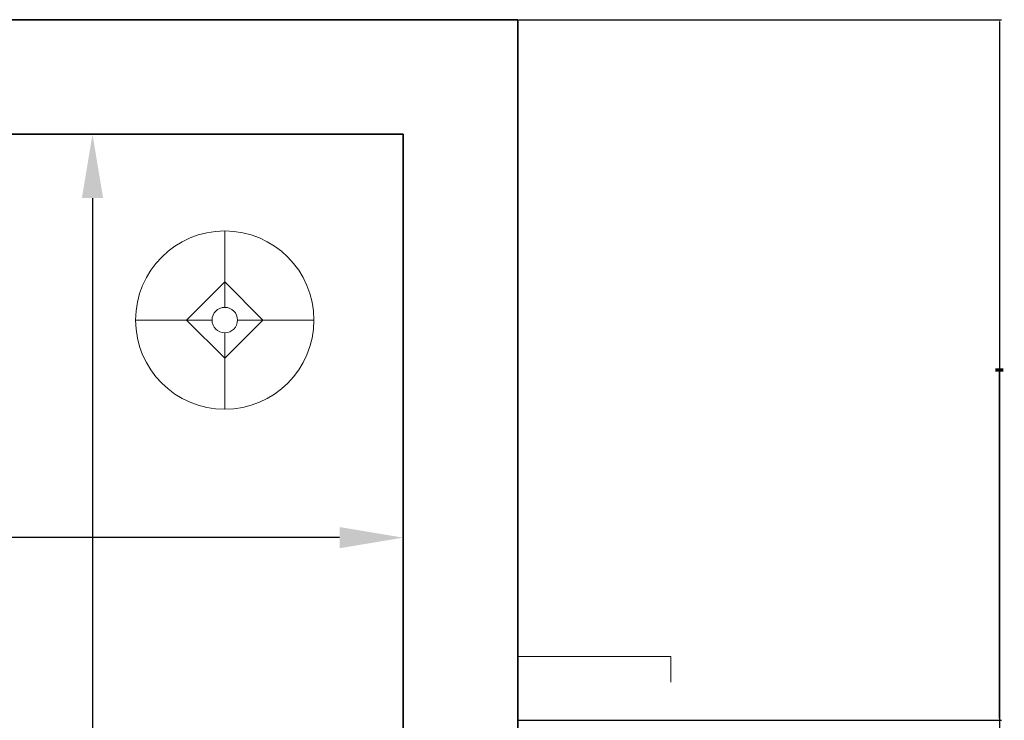
# Model space of a CAD drawing. Units: inches. Extents: x -128 to 854, y -395 to 398.
# Tile 49 of 61: x 275 to 352, y 294 to 349. Entities that reach past the tile are written whole.
import ezdxf

# ---------------------------------------------------------------- set-up
doc = ezdxf.new("R2010")
doc.units = ezdxf.units.IN
doc.header["$MEASUREMENT"] = 0
doc.linetypes.add('ACAD_ISO02W100', pattern=[15, 12, -3])
for name, color, linetype, lineweight in [('A-ANNO-DIMS', 2, 'Continuous', 18), ('A-FURN', 8, 'Continuous', 18), ('A-GLAZ-OVHD', 220, 'ACAD_ISO02W100', 13), ('A-WALL', 4, 'Continuous', 35)]:
    doc.layers.add(name, color=color, linetype=linetype, lineweight=lineweight)
doc.styles.get("Standard").update_dxf_attribs({"font": 'arial.ttf'})
doc.dimstyles.get("Standard").update_dxf_attribs({"dimtxt": 0.18, "dimasz": 0.18, "dimexe": 0.18, "dimexo": 0.0625, "dimgap": 0.09, "dimtad": 0, "dimtih": 1, "dimtoh": 1, "dimdec": 1, "dimzin": 0, "dimdsep": 46, "dimlunit": 4, "dimtxsty": 'Standard', "dimcen": 0.09, "dimclrd": 1, "dimclre": 2, "dimclrt": 6, "dimadec": 0, "dimazin": 0, "dimtfac": 1, "dimtdec": 1, "dimtofl": 0, "dimtmove": 0, "dimatfit": 3, "dimfxl": 1, "dimtfill": 2, "dimtfillclr": 3, "dimtolj": 1, "dimtzin": 0, "dimarcsym": 0})

# ---------------------------------------------------------------- blocks, each defined once
blk = doc.blocks.new('Lamp - Table')
for p, q in [((0, 7), (0, 1)), ((0, 3), (-3, 0)), ((3, 0), (0, 3)), ((-1, 0), (-7, 0)), ((-3, 0), (0, -3)), ((0, -3), (3, 0)), ((1, 0), (7, 0)), ((0, -1), (0, -7))]:
    blk.add_line(p, q)
for radius in [7, 1]:
    blk.add_circle((0, 0), radius)
blk = doc.blocks.new('*D52')
at = {"layer": 'A-ANNO-DIMS', "color": 0, "lineweight": -2, "transparency": 16777216}
for p, q in [((180.873, 339.678), (180.873, 307.9)), ((304.873, 339.678), (304.873, 307.9)), ((185.873, 308.08), (236.101, 308.08)), ((299.873, 308.08), (249.645, 308.08))]:
    blk.add_line(p, q, dxfattribs=at)
at = {"layer": 'A-ANNO-DIMS', "color": 0, "transparency": 16777216}
for points in [[(185.873, 308.913), (185.873, 307.247), (180.873, 308.08)], [(299.873, 308.913), (299.873, 307.247), (304.873, 308.08)]]:
    blk.add_solid(points, dxfattribs=at)
at = {"layer": 'Defpoints', "color": 0, "transparency": 16777216}
for p in [(180.873, 339.741), (304.873, 339.741), (304.873, 308.08)]:
    blk.add_point(p, dxfattribs=at)
at = {"layer": 'A-ANNO-DIMS', "color": 0, "transparency": 16777216, "insert": (242.873, 308.08), "char_height": 4, "attachment_point": 5, "bg_fill": 1, "box_fill_scale": 1.25, "bg_fill_color": 3, "bg_fill_transparency": 0}
blk.add_mtext('\\A1;10\'-4"', dxfattribs=at)
blk = doc.blocks.new('*D53')
at = {"layer": 'A-ANNO-DIMS', "color": 0, "lineweight": -2, "transparency": 16777216}
for p, q in [((304.81, 339.741), (280.297, 339.741)), ((280.477, 334.741), (280.477, 269.839)), ((280.477, 200.741), (280.477, 265.642)), ((304.81, 195.741), (280.297, 195.741))]:
    blk.add_line(p, q, dxfattribs=at)
at = {"layer": 'A-ANNO-DIMS', "color": 0, "transparency": 16777216}
for points in [[(279.644, 334.741), (281.311, 334.741), (280.477, 339.741)], [(279.644, 200.741), (281.311, 200.741), (280.477, 195.741)]]:
    blk.add_solid(points, dxfattribs=at)
at = {"layer": 'Defpoints', "color": 0, "transparency": 16777216}
for p in [(280.477, 339.741), (304.873, 339.741), (304.873, 195.741)]:
    blk.add_point(p, dxfattribs=at)
at = {"layer": 'A-ANNO-DIMS', "color": 0, "transparency": 16777216, "insert": (280.477, 267.741), "char_height": 4, "attachment_point": 5, "bg_fill": 1, "box_fill_scale": 1.25, "bg_fill_color": 3, "bg_fill_transparency": 0}
blk.add_mtext("\\A1;12'", dxfattribs=at)
blk = doc.blocks.new('SHADE-48IN')
at = {"ltscale": 2}
for p, q in [((12, 62), (0, 62)), ((0, 0), (0, 62)), ((12, 57), (12, 62)), ((12, 5), (12, 0)), ((12, 0), (0, 0))]:
    blk.add_line(p, q, dxfattribs=at)
blk = doc.blocks.new('*D98')
at = {"layer": 'A-ANNO-DIMS', "color": 2, "lineweight": -2, "transparency": 16777216}
for p, q in [((313.935, 348.741), (351.853, 348.741)), ((313.935, -89.259), (351.853, -89.259))]:
    blk.add_line(p, q, dxfattribs=at)
at = {"layer": 'A-ANNO-DIMS', "color": 1, "lineweight": -2, "transparency": 16777216}
for p, q in [((351.673, 348.561), (351.673, 129.923)), ((351.673, -89.079), (351.673, 129.559))]:
    blk.add_line(p, q, dxfattribs=at)
at = {"layer": 'A-ANNO-DIMS', "color": 1, "transparency": 16777216}
for points in [[(351.643, 348.561), (351.703, 348.561), (351.673, 348.741)], [(351.643, -89.079), (351.703, -89.079), (351.673, -89.259)]]:
    blk.add_solid(points, dxfattribs=at)
at = {"layer": 'Defpoints', "color": 0, "transparency": 16777216}
for p in [(313.873, 348.741), (351.673, 348.741), (313.873, -89.259)]:
    blk.add_point(p, dxfattribs=at)
at = {"layer": 'A-ANNO-DIMS', "color": 6, "transparency": 16777216, "insert": (351.673, 129.741), "char_height": 0.18, "attachment_point": 5, "bg_fill": 1, "box_fill_scale": 1.25, "bg_fill_color": 3, "bg_fill_transparency": 0}
blk.add_mtext('\\A1;36\'-6"', dxfattribs=at)
blk = doc.blocks.new('*D113')
at = {"layer": 'A-ANNO-DIMS', "color": 2, "lineweight": -2, "transparency": 16777216}
for p, q in [((313.935196, 348.740541), (351.852696, 348.740541)), ((313.935196, 293.740541), (351.852696, 293.740541))]:
    blk.add_line(p, q, dxfattribs=at)
at = {"layer": 'A-ANNO-DIMS', "color": 1, "lineweight": -2, "transparency": 16777216}
for p, q in [((351.672696, 348.560541), (351.672696, 321.420541)), ((351.672696, 293.920541), (351.672696, 321.060541))]:
    blk.add_line(p, q, dxfattribs=at)
at = {"layer": 'A-ANNO-DIMS', "color": 1, "transparency": 16777216}
for points in [[(351.642696, 348.560541), (351.702696, 348.560541), (351.672696, 348.740541)], [(351.642696, 293.920541), (351.702696, 293.920541), (351.672696, 293.740541)]]:
    blk.add_solid(points, dxfattribs=at)
at = {"layer": 'Defpoints', "color": 0, "transparency": 16777216}
for p in [(313.872696, 348.740541), (313.872696, 293.740541), (351.672696, 293.740541)]:
    blk.add_point(p, dxfattribs=at)
at = {"layer": 'A-ANNO-DIMS', "color": 6, "transparency": 16777216, "insert": (351.672696, 321.240541), "char_height": 0.18, "attachment_point": 5, "bg_fill": 1, "box_fill_scale": 1.25, "bg_fill_color": 3, "bg_fill_transparency": 0}
blk.add_mtext('\\A1;4\'-7"', dxfattribs=at)

msp = doc.modelspace()

# ---------------------------------------------------------------- linework, layer by layer
at = {"layer": 'A-WALL'}
for p, q in [((180.873, 348.741), (313.873, 348.741)), ((313.873, 348.741), (313.873, -89.259)), ((180.873, 339.741), (304.873, 339.741)), ((304.873, 339.741), (304.873, 195.741))]:
    msp.add_line(p, q, dxfattribs=at)

# ---------------------------------------------------------------- block references
at = {"layer": 'A-FURN'}
msp.add_blockref('Lamp - Table', (290.863, 325.158), dxfattribs=at)
at = {"layer": 'A-GLAZ-OVHD', "extrusion": (0, 0, -1), "zscale": -1}
msp.add_blockref('SHADE-48IN', (-325.873, 236.741), dxfattribs=at)

# ---------------------------------------------------------------- dimensions: what is measured, and where the dimension line sits
at = {"layer": 'A-ANNO-DIMS'}
for base, p1, p2, override, picture, middle in [((351.673, 348.741), (313.873, -89.259), (313.873, 348.741), {"dimdec": 1, "dimlfac": 1, "dimrnd": 0, "dimzin": 1, "dimdsep": 46, "dimlunit": 4, "dimfrac": 2}, '*D98', (351.673, 129.741)), ((351.673, 293.741), (313.873, 348.741), (313.873, 293.741), {"dimdec": 1, "dimlfac": 1, "dimrnd": 0, "dimzin": 1, "dimdsep": 46, "dimlunit": 4, "dimfrac": 2}, '*D113', (351.673, 321.241)), ((280.477, 339.741), (304.873, 195.741), (304.873, 339.741), {"dimtxt": 4, "dimasz": 5, "dimclrd": 0, "dimclre": 0, "dimclrt": 0}, '*D53', (280.477, 267.741))]:
    dim = msp.add_linear_dim(base=base, p1=p1, p2=p2, angle=90, dimstyle='Standard', override=override, dxfattribs=at)
    dim.commit()
    dim.dimension.update_dxf_attribs({"geometry": picture, "text_midpoint": middle})
dim = msp.add_linear_dim(base=(304.873, 308.08), p1=(180.873, 339.741), p2=(304.873, 339.741), dimstyle='Standard', override={"dimtxt": 4, "dimasz": 5, "dimclrd": 0, "dimclre": 0, "dimclrt": 0}, dxfattribs=at)
dim.commit()
dim.dimension.update_dxf_attribs({"geometry": '*D52', "text_midpoint": (242.873, 308.08)})

doc.saveas('drawing.dxf')
